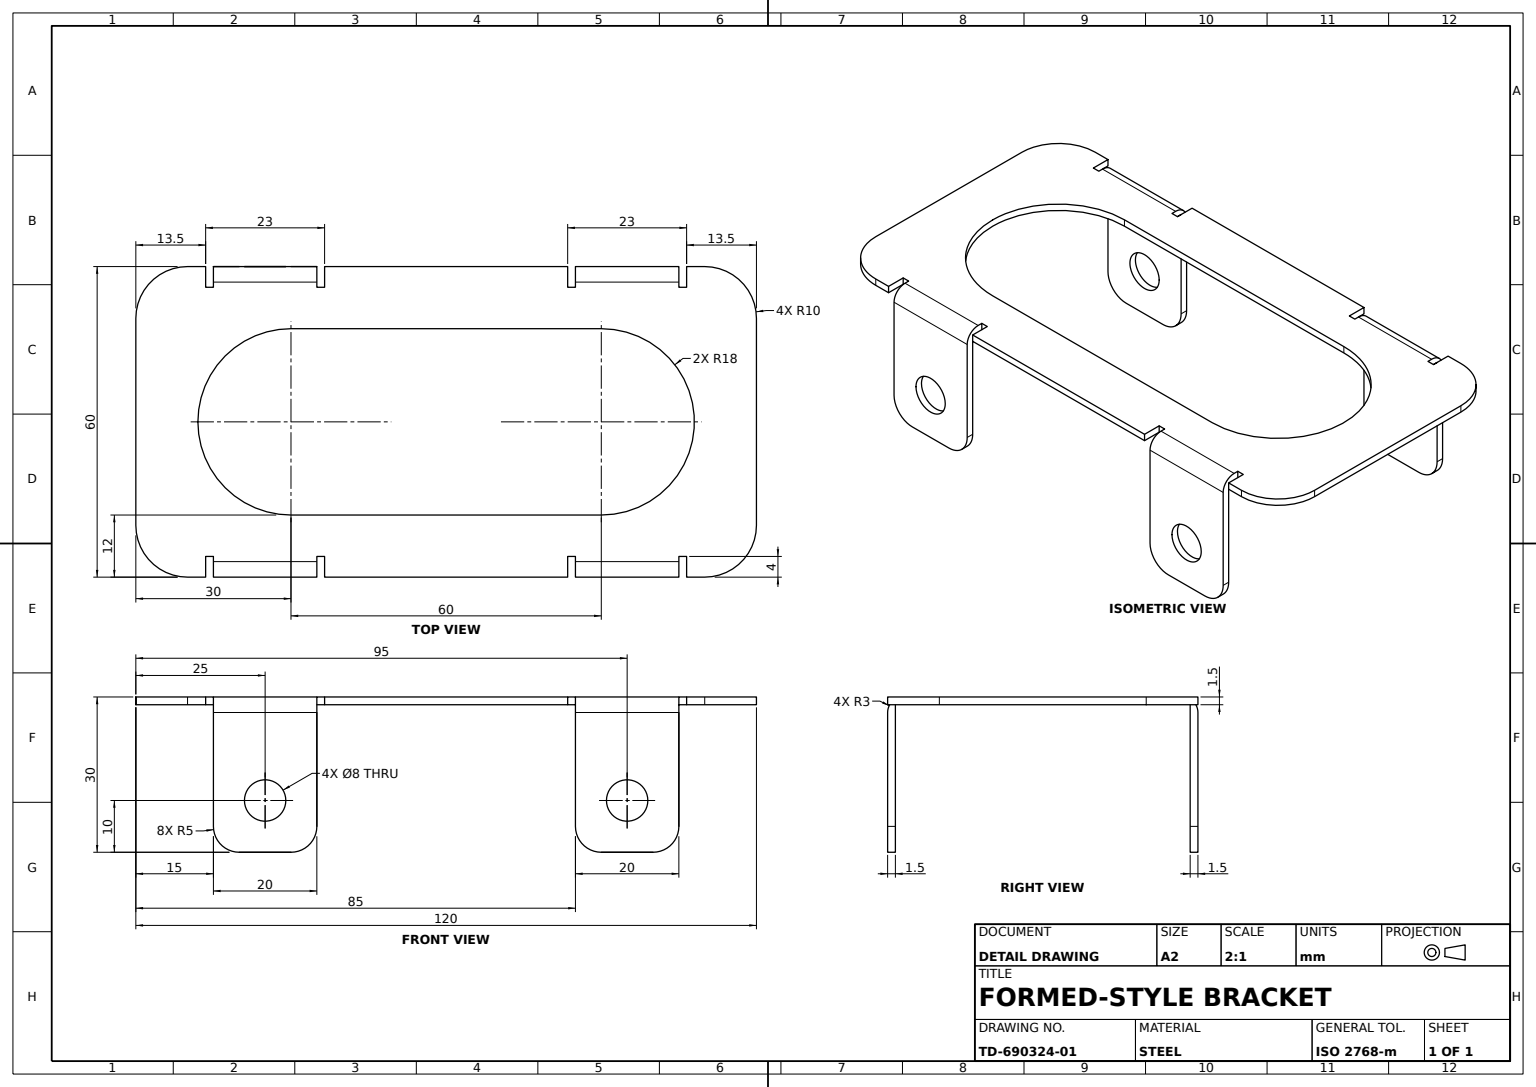
SolidWorks part; units mm, degrees
material "Plain Carbon Steel"
ref_plane "Front Plane" through (0, 0, 0) normal (0, 0, 1) x (1, 0, 0)
ref_plane "Top Plane" through (0, 0, 0) normal (0, 1, 0) x (1, 0, 0)
ref_plane "Right Plane" through (0, 0, 0) normal (1, 0, 0) x (0, 0, -1)
sketch "Cover Plate Sketch" plane through (0, 0, 0) normal (0, 1, 0) x (1, 0, 0)
  line L0 (-30, 45) -> (-26, 45)
  line L1 (-20, 60) -> (20, 60)
  line L2 (-30, 50) -> (-30, 46.5)
  line L3 (-20, -60) -> (20, -60)
  line L4 (30, 50) -> (30, 46.5)
  line L5 (-30, 60) -> (30, -60) construction
  line L6 (-30, -60) -> (30, 60) construction
  line L7 (-30, -45) -> (-26, -45)
  line L8 (-30, -46.5) -> (-26, -46.5)
  line L9 (-30, 46.5) -> (-26, 46.5)
  line L10 (-26, 46.5) -> (-26, 45)
  line L11 (-30, 45) -> (-30, 25)
  line L12 (26, 46.5) -> (30, 46.5)
  line L13 (-26, 60) -> (-26, -60) construction
  line L14 (26, 45) -> (30, 45)
  line L15 (-30, 46.5) -> (30, 46.5) construction
  line L16 (-26, -45) -> (-26, -46.5)
  line L17 (-30, 45) -> (30, 45) construction
  line L18 (26, -45) -> (30, -45)
  line L19 (26, -46.5) -> (30, -46.5)
  line L20 (-30, -45) -> (30, -45) construction
  line L21 (30, -46.5) -> (30, -50)
  line L22 (-30, -46.5) -> (30, -46.5) construction
  line L23 (26, -45) -> (26, -46.5)
  line L24 (30, 45) -> (30, 25)
  line L25 (-30, -46.5) -> (-30, -50)
  line L26 (-30, 25) -> (-26, 25)
  line L27 (26, 46.5) -> (26, 45)
  line L28 (-30, 60) -> (-30, -60) construction
  line L29 (-30, -25) -> (-26, -25)
  line L30 (-30, 23.5) -> (-26, 23.5)
  line L31 (-30, -23.5) -> (-26, -23.5)
  line L32 (-26, 25) -> (-26, 23.5)
  line L33 (26, 25) -> (26, 23.5)
  line L34 (26, 25) -> (30, 25)
  line L35 (-26, 45) -> (-26, -45) construction
  line L36 (26, 23.5) -> (30, 23.5)
  line L37 (-30, 25) -> (30, 25) construction
  line L38 (-26, -23.5) -> (-26, -25)
  line L39 (-30, 23.5) -> (30, 23.5) construction
  line L40 (-30, 23.5) -> (-30, -23.5)
  line L41 (26, -23.5) -> (26, -25)
  line L42 (-30, 45) -> (-30, -45) construction
  line L43 (26, 45) -> (26, -45) construction
  line L44 (30, 23.5) -> (30, -23.5)
  line L45 (30, -25) -> (30, -45)
  line L46 (30, 45) -> (30, -45) construction
  line L47 (-30, -25) -> (-30, -45)
  line L48 (-30, -23.5) -> (30, -23.5) construction
  line L49 (26, -23.5) -> (30, -23.5)
  line L50 (-30, -25) -> (30, -25) construction
  line L51 (26, -25) -> (30, -25)
  line L52 (-30, -60) -> (30, -60) construction
  line L53 (-30, 60) -> (30, 60) construction
  arc A0 (-30, -50) -> (-20, -60) centre (-20, -50) ccw
  arc A1 (20, -60) -> (30, -50) centre (20, -50) ccw
  arc A2 (20, 60) -> (30, 50) centre (20, 50) cw
  arc A3 (-20, 60) -> (-30, 50) centre (-20, 50) ccw
  point P0 (0, 0)
  point P16 (30, 60)
  dimension "D11" = 10
  dimension "D1" = 60
  dimension "D2" = 120
  dimension "D8" = 4
  dimension "D3" = 20
  dimension "D4" = 4
  dimension "D5" = 23.5
  dimension "D6" = 23.5
  dimension "D7" = 20
  dimension "D10" = 1.5
  dimension "D12" = 1.5
  dimension "D13" = 1.5
  dimension "D9" = 4
extrude "Cover Plate 1.5mm" add sketch "Cover Plate Sketch" along normal blind 1.5
sketch "Side A Legs Sketch" plane through (30, 0, 0) normal (1, 0, 0) x (0, 0, -1)
  line L1 (-45, 1.5) -> (-25, 1.5)
  line L2 (-45, 1.5) -> (-45, -23.5)
  line L3 (-40, -28.5) -> (-30, -28.5)
  line L4 (-25, 1.5) -> (-25, -23.5)
  line L5 (25, 1.5) -> (45, 1.5)
  line L6 (25, 1.5) -> (25, -23.5)
  line L7 (30, -28.5) -> (40, -28.5)
  line L8 (45, 1.5) -> (45, -23.5)
  arc A0 (40, -28.5) -> (45, -23.5) centre (40, -23.5) ccw
  arc A1 (25, -23.5) -> (30, -28.5) centre (30, -23.5) ccw
  arc A2 (-30, -28.5) -> (-25, -23.5) centre (-30, -23.5) ccw
  arc A3 (-45, -23.5) -> (-40, -28.5) centre (-40, -23.5) ccw
  circle A4 centre (-35, -18.5) radius 4
  circle A5 centre (35, -18.5) radius 4
  point P18 (-45, -28.5)
  point P24 (-35, -28.5)
  point P26 (35, -28.5)
  dimension "D5" = 5
  dimension "D6" = 10
  dimension "D8" = 8
  dimension "D9" = 8
  dimension "D1" = 30
  dimension "D2" = 20
  dimension "D3" = 20
  dimension "D4" = 30
  dimension "D7" = 10
extrude "Side A Mounting Legs" add sketch "Side A Legs Sketch" against normal blind 1.5
sketch "Side B Legs Sketch" plane through (-30, 0, 0) normal (-1, 0, 0) x (0, 0, 1)
  line L1 (-45, 1.5) -> (-25, 1.5)
  line L2 (-45, 1.5) -> (-45, -23.5)
  line L3 (-40, -28.5) -> (-30, -28.5)
  line L4 (-25, 1.5) -> (-25, -23.5)
  line L5 (25, 1.5) -> (45, 1.5)
  line L6 (25, 1.5) -> (25, -23.5)
  line L7 (30, -28.5) -> (40, -28.5)
  line L8 (45, 1.5) -> (45, -23.5)
  arc A0 (40, -28.5) -> (45, -23.5) centre (40, -23.5) ccw
  arc A1 (25, -23.5) -> (30, -28.5) centre (30, -23.5) ccw
  arc A2 (-30, -28.5) -> (-25, -23.5) centre (-30, -23.5) ccw
  arc A3 (-45, -23.5) -> (-40, -28.5) centre (-40, -23.5) ccw
  circle A4 centre (-35, -18.5) radius 4
  circle A5 centre (35, -18.5) radius 4
  point P12 (45, -28.5)
  point P15 (25, -28.5)
  point P18 (-25, -28.5)
  point P21 (-45, -28.5)
  dimension "D5" = 5
  dimension "D6" = 8
  dimension "D7" = 8
  dimension "D1" = 30
  dimension "D2" = 20
  dimension "D3" = 30
  dimension "D4" = 20
extrude "Side B Mounting Legs" add sketch "Side B Legs Sketch" against normal blind 1.5
fillet "Corner Fillets R3" radius 3 4 edges at (30, 1.5, 35) (30, 1.5, -35) (-30, 1.5, 35) (-30, 1.5, -35)
sketch "Oblong Slot Sketch" plane through (0, 1.5, 0) normal (0, 1, 0) x (1, 0, 0)
  line L1 (0, -30) -> (0, 30) construction
  line L2 (-18, -30) -> (-18, 30)
  line L3 (18, -30) -> (18, 30)
  line L9 (-30, 23.5) -> (-30, -23.5) construction
  arc A0 (-18, -30) -> (18, -30) centre (0, -30) ccw
  arc A1 (18, 30) -> (-18, 30) centre (0, 30) ccw
  point P0 (0, 0)
  point P4 (0, 0)
  dimension "D2" = 18
  dimension "D1" = 60
  dimension "D3" = 12
extrude "Oblong Slot Cut" cut sketch "Oblong Slot Sketch" against normal blind 1.5
